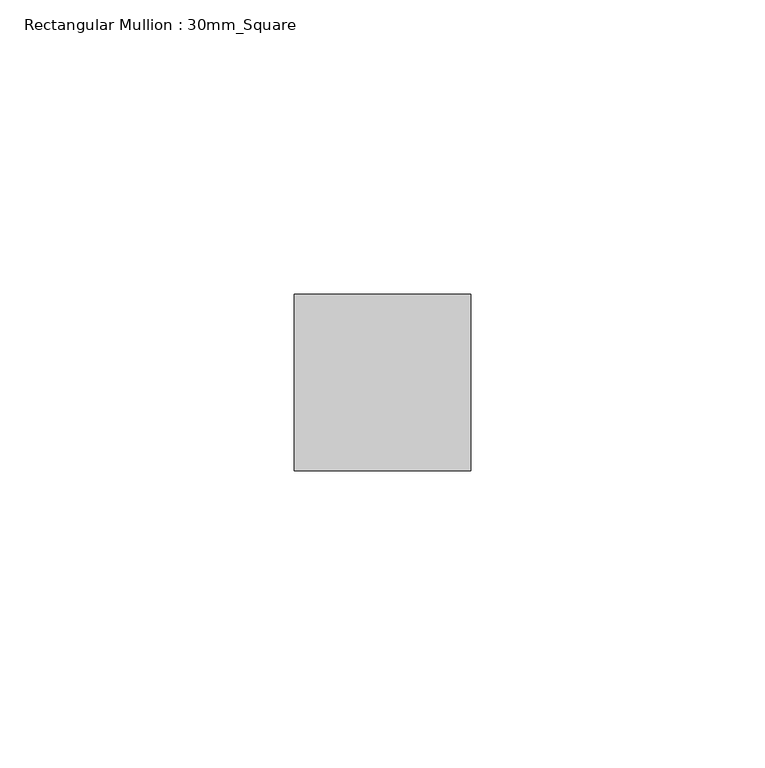
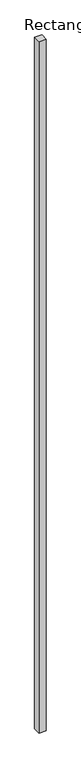
"""IFC4 building model written with IfcOpenShell, lengths in millimetres: member geometry, Rectangular Mullion : 30mm_Square."""

from ifc_helpers import new_model, si_unit, frame, origin, place, context, project, spatial, polyline, outline, extrude, source, transform, mapped, element, save


def rectangular_mullion_30mm_square_0acd70fe(model_context):
    return source(origin(), model_context, "Body", "SweptSolid", [
        extrude(outline(polyline([(0.0, 15.0), (0.0, -15.0), (-30.0, -15.0), (-30.0, 15.0), (0.0, 15.0)])), frame((0.0, 0.0, -3000.0), z_axis=(0.0, 0.0, 1.0), x_axis=(1.0, 0.0, 0.0)), (0.0, 0.0, 1.0), 3000.0),
    ])


if __name__ == "__main__":
    model = new_model("IFC4")
    model_context = context("Model", 3, world=origin())
    ifc_project = project(units=[si_unit("LENGTHUNIT", "METRE", prefix="MILLI")], contexts=[model_context])
    site = spatial("IfcSite", under=ifc_project)
    building = spatial("IfcBuilding", under=site)
    placement = place(None, origin())
    rectangular_mullion_30mm_square_shape = rectangular_mullion_30mm_square_0acd70fe(model_context)
    element("IfcMember", 1, ObjectType="Rectangular Mullion : 30mm_Square", at=placement, inside=building, context=model_context, shape_type="MappedRepresentation", body=[
        mapped(rectangular_mullion_30mm_square_shape, transform((0.0, 0.0, 0.0), x_axis=(1.0, 0.0, 0.0), y_axis=(0.0, 1.0, 0.0), z_axis=(0.0, 0.0, 1.0))),
    ])
    save(model, "model.ifc")

# Revit data of these elements
# Type "Rectangular Mullion : 30mm_Square"
#   Keynote = "H11"
#   built-in parameter 1007304 = 0.0984252 (stored number, unit not read)
#   built-in parameter 1007301 = 0.0492126 (stored number, unit not read)
#   built-in parameter 1007300 = 0.0492126 (stored number, unit not read)
# Element 1 (IfcMember, "Rectangular Mullion : 30mm_Square")
#   Materials on its faces: "Aluminium"
# Materials
#   "Aluminium": class "Metal", colour RGB 247 247 247, transparency 0, Description = "Aluminium 6061", Cost = 0
